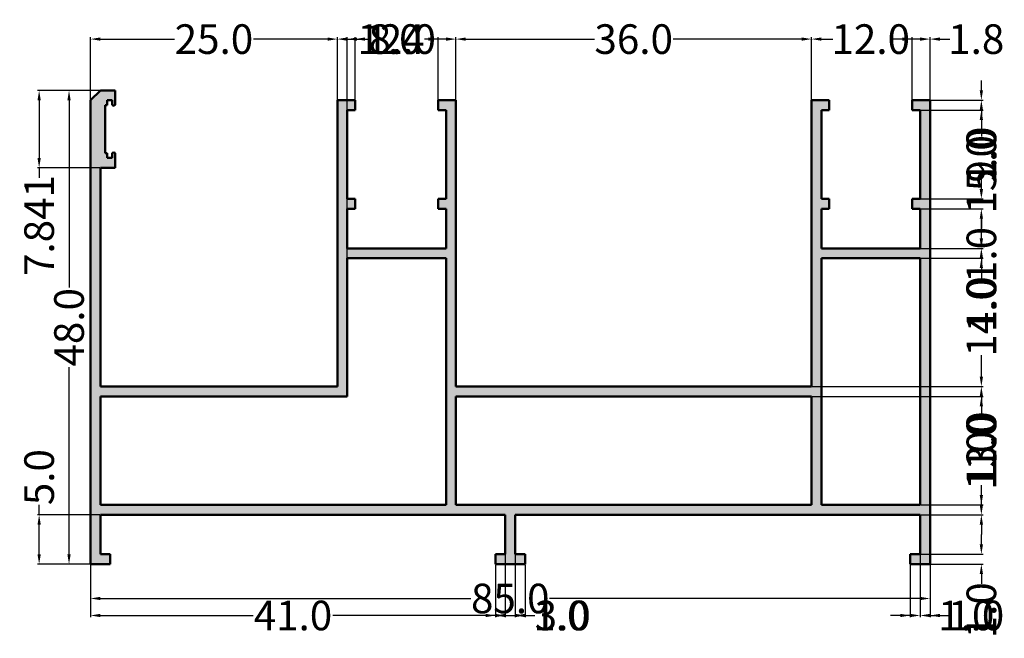
# Model space of a CAD drawing. Units: millimetres. Extents: x 9 to 262, y -226 to 104.
# Tile 2 of 4: x 9 to 109, y 42 to 104. Entities that reach past the tile are written whole.
import ezdxf

# ---------------------------------------------------------------- set-up
doc = ezdxf.new("R2010")
doc.units = ezdxf.units.MM
doc.header["$MEASUREMENT"] = 0
for name, color, linetype, lineweight in [('M-DIMS', 2, 'Continuous', 25), ('M-HATC', 9, 'Continuous', 18), ('M-OUTL', 7, 'Continuous', 50)]:
    doc.layers.add(name, color=color, linetype=linetype, lineweight=lineweight)
doc.styles.get("Standard").update_dxf_attribs({"font": 'arial.ttf'})
doc.dimstyles.get("Standard").update_dxf_attribs({"dimtxt": 3, "dimasz": 1, "dimexe": 0.18, "dimexo": 0.0625, "dimgap": 0.09, "dimtad": 0, "dimdec": 1, "dimzin": 0, "dimdsep": 46, "dimtxsty": 'Standard', "dimcen": 0.09, "dimadec": 0, "dimazin": 0, "dimtfac": 1, "dimtdec": 1, "dimtofl": 0, "dimtmove": 0, "dimatfit": 3, "dimfxl": 1, "dimtolj": 1, "dimtzin": 0, "dimarcsym": 0})

# ---------------------------------------------------------------- blocks, each defined once
blk = doc.blocks.new('*D1')
at = {"layer": 'Defpoints', "color": 0, "transparency": 16777216}
for p in [(17.228, 97.071), (14.054, 49.071), (17.228, 49.071)]:
    blk.add_point(p, dxfattribs=at)
at = {"layer": 'M-DIMS', "color": 0, "lineweight": -2, "transparency": 16777216}
for p, q in [((17.166, 97.071), (13.874, 97.071)), ((14.054, 96.071), (14.054, 77.112)), ((14.054, 50.071), (14.054, 69.029)), ((17.166, 49.071), (13.874, 49.071))]:
    blk.add_line(p, q, dxfattribs=at)
at = {"layer": 'M-DIMS', "color": 0, "transparency": 16777216}
for points in [[(13.888, 96.071), (14.221, 96.071), (14.054, 97.071)], [(13.888, 50.071), (14.221, 50.071), (14.054, 49.071)]]:
    blk.add_solid(points, dxfattribs=at)
at = {"layer": 'M-DIMS', "color": 0, "transparency": 16777216, "insert": (14.054, 73.071), "char_height": 3, "attachment_point": 5, "rotation": 90}
blk.add_mtext('\\A1;48.0', dxfattribs=at)
blk = doc.blocks.new('*D2')
at = {"layer": 'Defpoints', "color": 0, "transparency": 16777216}
for p in [(16.228, 49.071), (101.228, 49.071), (101.228, 45.592)]:
    blk.add_point(p, dxfattribs=at)
at = {"layer": 'M-DIMS', "color": 0, "lineweight": -2, "transparency": 16777216}
for p, q in [((16.228, 49.008), (16.228, 45.412)), ((101.228, 49.008), (101.228, 45.412)), ((17.228, 45.592), (54.745, 45.592)), ((100.228, 45.592), (62.711, 45.592))]:
    blk.add_line(p, q, dxfattribs=at)
at = {"layer": 'M-DIMS', "color": 0, "transparency": 16777216}
for points in [[(17.228, 45.759), (17.228, 45.426), (16.228, 45.592)], [(100.228, 45.759), (100.228, 45.426), (101.228, 45.592)]]:
    blk.add_solid(points, dxfattribs=at)
at = {"layer": 'M-DIMS', "color": 0, "transparency": 16777216, "insert": (58.728, 45.592), "char_height": 3, "attachment_point": 5}
blk.add_mtext('\\A1;85.0', dxfattribs=at)
blk = doc.blocks.new('PROFILE-FRAME')
for p, q in [((0, 47), (1, 48)), ((1, 48), (2.5, 48)), ((2.5, 48), (2.5, 46.6)), ((0, 47), (0, 0)), ((1.7, 47), (2.2, 47)), ((1.7, 47), (2.2, 47)), ((2.2, 47), (1.7, 47)), ((1.7, 47), (1.7, 46.5)), ((2.2, 46.6), (2.2, 47)), ((25, 47), (25, 18)), ((25, 47), (26.8, 47)), ((26.8, 47), (26.8, 46)), ((36, 47), (35.2, 47)), ((35.2, 47), (35.2, 46)), ((35.2, 47), (37, 47)), ((37, 47), (37, 18)), ((73, 47), (73, 18)), ((73, 47), (74.8, 47)), ((74, 47), (74.8, 47)), ((74.8, 47), (74.8, 46)), ((84, 47), (83.2, 47)), ((83.2, 47), (83.2, 46)), ((83.2, 47), (85, 47)), ((85, 47), (85, 0)), ((1.5, 46.5), (1.5, 41.659)), ((1.7, 46.5), (1.5, 46.5)), ((26, 46), (26, 37)), ((26, 46), (26.8, 46)), ((35.2, 46), (36, 46)), ((35.2, 46), (36, 46)), ((36, 46), (36, 37)), ((74, 46), (74, 37)), ((74, 46), (74.8, 46)), ((83.2, 46), (84, 46)), ((84, 46), (84, 37)), ((1.7, 41.659), (1.5, 41.659)), ((1.7, 41.159), (1.7, 41.659)), ((1.7, 41.159), (2.2, 41.159)), ((1.7, 41.159), (2.2, 41.159)), ((2.2, 41.159), (1.7, 41.159)), ((2.2, 41.559), (2.2, 41.159)), ((2.5, 40.159), (2.5, 41.559)), ((1, 40.159), (2.5, 40.159)), ((1, 40.159), (1, 18)), ((26, 37), (26.8, 37)), ((26.8, 37), (26.8, 36)), ((35.2, 37), (36, 37)), ((35.2, 37), (36, 37)), ((35.2, 37), (35.2, 36)), ((74, 37), (74.8, 37)), ((74.8, 37), (74.8, 36)), ((83.2, 37), (84, 37)), ((83.2, 37), (83.2, 36)), ((26, 36), (26.8, 36)), ((26, 36), (26, 33)), ((35.2, 36), (36, 36)), ((36, 36), (36, 33)), ((74, 36), (74.8, 36)), ((74, 36), (74, 33)), ((83.2, 36), (84, 36)), ((84, 36), (84, 33)), ((26, 33), (26, 32)), ((36, 33), (36, 32)), ((74, 33), (74, 32)), ((84, 33), (84, 32)), ((26, 32), (36, 32)), ((74, 32), (84, 32)), ((26, 31), (36, 31)), ((26, 31), (26, 27)), ((36, 31), (36, 27)), ((74, 31), (84, 31)), ((74, 31), (74, 27)), ((84, 31), (84, 27)), ((26, 27), (26, 17)), ((36, 27), (36, 6)), ((74, 27), (74, 17)), ((84, 27), (84, 17)), ((1, 18), (25, 18)), ((37, 18), (73, 18)), ((1, 17), (26, 17)), ((1, 17), (1, 6)), ((37, 17), (73, 17)), ((37, 17), (37, 6)), ((73, 17), (73, 6)), ((74, 17), (74, 6)), ((84, 17), (84, 6)), ((1, 6), (36, 6)), ((37, 6), (73, 6)), ((74, 6), (84, 6)), ((1, 5), (42, 5)), ((1, 5), (1, 1)), ((42, 5), (42, 1)), ((43, 5), (43, 1)), ((43, 5), (84, 5)), ((84, 5), (84, 1)), ((1, 1), (2, 1)), ((1, 1), (2, 1)), ((2, 1), (2, 0)), ((41, 1), (42, 1)), ((41, 1), (41, 0)), ((43, 1), (44, 1)), ((43, 1), (44, 1)), ((44, 1), (44, 0)), ((84, 1), (83, 1)), ((83, 1), (83, 0)), ((83, 1), (84, 1)), ((0, 0), (2, 0)), ((41, 0), (44, 0)), ((83, 0), (85, 0))]:
    blk.add_line(p, q)
for centre, start, end in [((2.35, 46.6), 180, 0), ((2.35, 41.559), 0, 180)]:
    blk.add_arc(centre, 0.15, start, end)
blk = doc.blocks.new('*D7')
at = {"layer": 'Defpoints', "color": 0, "transparency": 16777216}
for p in [(41.228, 102.271), (16.228, 96.071), (41.228, 96.071)]:
    blk.add_point(p, dxfattribs=at)
at = {"layer": 'M-DIMS', "color": 0, "lineweight": -2, "transparency": 16777216}
for p, q in [((16.228, 96.133), (16.228, 102.451)), ((17.228, 102.271), (24.721, 102.271)), ((40.228, 102.271), (32.735, 102.271)), ((41.228, 96.133), (41.228, 102.451))]:
    blk.add_line(p, q, dxfattribs=at)
at = {"layer": 'M-DIMS', "color": 0, "transparency": 16777216}
for points in [[(17.228, 102.438), (17.228, 102.104), (16.228, 102.271)], [(40.228, 102.438), (40.228, 102.104), (41.228, 102.271)]]:
    blk.add_solid(points, dxfattribs=at)
at = {"layer": 'M-DIMS', "color": 0, "transparency": 16777216, "insert": (28.728, 102.271), "char_height": 3, "attachment_point": 5}
blk.add_mtext('\\A1;25.0', dxfattribs=at)
blk = doc.blocks.new('*D8')
at = {"layer": 'Defpoints', "color": 0, "transparency": 16777216}
for p in [(53.228, 102.271), (41.228, 96.071), (53.228, 96.071)]:
    blk.add_point(p, dxfattribs=at)
at = {"layer": 'M-DIMS', "color": 0, "lineweight": -2, "transparency": 16777216}
for p, q in [((41.228, 96.133), (41.228, 102.451)), ((42.228, 102.271), (43.388, 102.271)), ((52.228, 102.271), (51.068, 102.271)), ((53.228, 96.133), (53.228, 102.451))]:
    blk.add_line(p, q, dxfattribs=at)
at = {"layer": 'M-DIMS', "color": 0, "transparency": 16777216}
for points in [[(42.228, 102.438), (42.228, 102.104), (41.228, 102.271)], [(52.228, 102.438), (52.228, 102.104), (53.228, 102.271)]]:
    blk.add_solid(points, dxfattribs=at)
at = {"layer": 'M-DIMS', "color": 0, "transparency": 16777216, "insert": (47.228, 102.271), "char_height": 3, "attachment_point": 5}
blk.add_mtext('\\A1;12.0', dxfattribs=at)
blk = doc.blocks.new('*D9')
at = {"layer": 'Defpoints', "color": 0, "transparency": 16777216}
for p in [(89.228, 102.271), (53.228, 96.071), (89.228, 96.071)]:
    blk.add_point(p, dxfattribs=at)
at = {"layer": 'M-DIMS', "color": 0, "lineweight": -2, "transparency": 16777216}
for p, q in [((53.228, 96.133), (53.228, 102.451)), ((54.228, 102.271), (67.248, 102.271)), ((88.228, 102.271), (75.208, 102.271)), ((89.228, 96.133), (89.228, 102.451))]:
    blk.add_line(p, q, dxfattribs=at)
at = {"layer": 'M-DIMS', "color": 0, "transparency": 16777216}
for points in [[(54.228, 102.438), (54.228, 102.104), (53.228, 102.271)], [(88.228, 102.438), (88.228, 102.104), (89.228, 102.271)]]:
    blk.add_solid(points, dxfattribs=at)
at = {"layer": 'M-DIMS', "color": 0, "transparency": 16777216, "insert": (71.228, 102.271), "char_height": 3, "attachment_point": 5}
blk.add_mtext('\\A1;36.0', dxfattribs=at)
blk = doc.blocks.new('*D10')
at = {"layer": 'Defpoints', "color": 0, "transparency": 16777216}
for p in [(101.228, 102.271), (89.228, 96.071), (101.228, 96.071)]:
    blk.add_point(p, dxfattribs=at)
at = {"layer": 'M-DIMS', "color": 0, "lineweight": -2, "transparency": 16777216}
for p, q in [((89.228, 96.133), (89.228, 102.451)), ((90.228, 102.271), (91.388, 102.271)), ((100.228, 102.271), (99.068, 102.271)), ((101.228, 96.133), (101.228, 102.451))]:
    blk.add_line(p, q, dxfattribs=at)
at = {"layer": 'M-DIMS', "color": 0, "transparency": 16777216}
for points in [[(90.228, 102.438), (90.228, 102.104), (89.228, 102.271)], [(100.228, 102.438), (100.228, 102.104), (101.228, 102.271)]]:
    blk.add_solid(points, dxfattribs=at)
at = {"layer": 'M-DIMS', "color": 0, "transparency": 16777216, "insert": (95.228, 102.271), "char_height": 3, "attachment_point": 5}
blk.add_mtext('\\A1;12.0', dxfattribs=at)
blk = doc.blocks.new('*D11')
at = {"layer": 'Defpoints', "color": 0, "transparency": 16777216}
for p in [(11.028, 54.071), (17.228, 54.071), (16.228, 49.071)]:
    blk.add_point(p, dxfattribs=at)
at = {"layer": 'M-DIMS', "color": 0, "lineweight": -2, "transparency": 16777216}
for p, q in [((11.028, 54.071), (11.028, 55.071)), ((17.166, 54.071), (10.848, 54.071)), ((11.028, 50.071), (11.028, 53.071)), ((16.166, 49.071), (10.848, 49.071))]:
    blk.add_line(p, q, dxfattribs=at)
at = {"layer": 'M-DIMS', "color": 0, "transparency": 16777216}
for points in [[(10.861, 53.071), (11.195, 53.071), (11.028, 54.071)], [(10.861, 50.071), (11.195, 50.071), (11.028, 49.071)]]:
    blk.add_solid(points, dxfattribs=at)
at = {"layer": 'M-DIMS', "color": 0, "transparency": 16777216, "insert": (11.028, 57.887), "char_height": 3, "attachment_point": 5, "rotation": 90}
blk.add_mtext('\\A1;5.0', dxfattribs=at)
blk = doc.blocks.new('*D12')
at = {"layer": 'Defpoints', "color": 0, "transparency": 16777216}
for p in [(89.228, 67.071), (106.428, 67.071), (100.228, 54.071)]:
    blk.add_point(p, dxfattribs=at)
at = {"layer": 'M-DIMS', "color": 0, "lineweight": -2, "transparency": 16777216}
for p, q in [((89.291, 67.071), (106.608, 67.071)), ((106.428, 66.071), (106.428, 64.411)), ((106.428, 55.071), (106.428, 56.731)), ((100.291, 54.071), (106.608, 54.071))]:
    blk.add_line(p, q, dxfattribs=at)
at = {"layer": 'M-DIMS', "color": 0, "transparency": 16777216}
for points in [[(106.261, 66.071), (106.595, 66.071), (106.428, 67.071)], [(106.261, 55.071), (106.595, 55.071), (106.428, 54.071)]]:
    blk.add_solid(points, dxfattribs=at)
at = {"layer": 'M-DIMS', "color": 0, "transparency": 16777216, "insert": (106.428, 60.571), "char_height": 3, "attachment_point": 5, "rotation": 90}
blk.add_mtext('\\A1;13.0', dxfattribs=at)
blk = doc.blocks.new('*D13')
at = {"layer": 'Defpoints', "color": 0, "transparency": 16777216}
for p in [(90.228, 81.071), (106.428, 81.071), (89.228, 67.071)]:
    blk.add_point(p, dxfattribs=at)
at = {"layer": 'M-DIMS', "color": 0, "lineweight": -2, "transparency": 16777216}
for p, q in [((90.291, 81.071), (106.608, 81.071)), ((106.428, 80.071), (106.428, 77.911)), ((106.428, 68.071), (106.428, 70.231)), ((89.291, 67.071), (106.608, 67.071))]:
    blk.add_line(p, q, dxfattribs=at)
at = {"layer": 'M-DIMS', "color": 0, "transparency": 16777216}
for points in [[(106.261, 80.071), (106.595, 80.071), (106.428, 81.071)], [(106.261, 68.071), (106.595, 68.071), (106.428, 67.071)]]:
    blk.add_solid(points, dxfattribs=at)
at = {"layer": 'M-DIMS', "color": 0, "transparency": 16777216, "insert": (106.428, 74.071), "char_height": 3, "attachment_point": 5, "rotation": 90}
blk.add_mtext('\\A1;14.0', dxfattribs=at)
blk = doc.blocks.new('*D14')
at = {"layer": 'Defpoints', "color": 0, "transparency": 16777216}
for p in [(101.228, 96.071), (106.428, 96.071), (90.228, 81.071)]:
    blk.add_point(p, dxfattribs=at)
at = {"layer": 'M-DIMS', "color": 0, "lineweight": -2, "transparency": 16777216}
for p, q in [((101.291, 96.071), (106.608, 96.071)), ((106.428, 95.071), (106.428, 92.411)), ((106.428, 82.071), (106.428, 84.731)), ((90.291, 81.071), (106.608, 81.071))]:
    blk.add_line(p, q, dxfattribs=at)
at = {"layer": 'M-DIMS', "color": 0, "transparency": 16777216}
for points in [[(106.261, 95.071), (106.595, 95.071), (106.428, 96.071)], [(106.261, 82.071), (106.595, 82.071), (106.428, 81.071)]]:
    blk.add_solid(points, dxfattribs=at)
at = {"layer": 'M-DIMS', "color": 0, "transparency": 16777216, "insert": (106.428, 88.571), "char_height": 3, "attachment_point": 5, "rotation": 90}
blk.add_mtext('\\A1;15.0', dxfattribs=at)
blk = doc.blocks.new('*D15')
at = {"layer": 'Defpoints', "color": 0, "transparency": 16777216}
for p in [(16.228, 49.071), (57.228, 49.071), (57.228, 43.871)]:
    blk.add_point(p, dxfattribs=at)
at = {"layer": 'M-DIMS', "color": 0, "lineweight": -2, "transparency": 16777216}
for p, q in [((16.228, 49.008), (16.228, 43.691)), ((57.228, 49.008), (57.228, 43.691)), ((17.228, 43.871), (32.687, 43.871)), ((56.228, 43.871), (40.77, 43.871))]:
    blk.add_line(p, q, dxfattribs=at)
at = {"layer": 'M-DIMS', "color": 0, "transparency": 16777216}
for points in [[(17.228, 44.038), (17.228, 43.704), (16.228, 43.871)], [(56.228, 44.038), (56.228, 43.704), (57.228, 43.871)]]:
    blk.add_solid(points, dxfattribs=at)
at = {"layer": 'M-DIMS', "color": 0, "transparency": 16777216, "insert": (36.728, 43.871), "char_height": 3, "attachment_point": 5}
blk.add_mtext('\\A1;41.0', dxfattribs=at)
blk = doc.blocks.new('*D16')
at = {"layer": 'Defpoints', "color": 0, "transparency": 16777216}
for p in [(57.228, 49.071), (60.228, 49.071), (60.228, 43.871)]:
    blk.add_point(p, dxfattribs=at)
at = {"layer": 'M-DIMS', "color": 0, "lineweight": -2, "transparency": 16777216}
for p, q in [((57.228, 49.008), (57.228, 43.691)), ((60.228, 49.008), (60.228, 43.691)), ((58.228, 43.871), (59.228, 43.871)), ((60.228, 43.871), (61.228, 43.871))]:
    blk.add_line(p, q, dxfattribs=at)
at = {"layer": 'M-DIMS', "color": 0, "transparency": 16777216}
for points in [[(58.228, 44.038), (58.228, 43.704), (57.228, 43.871)], [(59.228, 44.038), (59.228, 43.704), (60.228, 43.871)]]:
    blk.add_solid(points, dxfattribs=at)
at = {"layer": 'M-DIMS', "color": 0, "transparency": 16777216, "insert": (64.043, 43.871), "char_height": 3, "attachment_point": 5}
blk.add_mtext('\\A1;3.0', dxfattribs=at)
blk = doc.blocks.new('*D17')
at = {"layer": 'Defpoints', "color": 0, "transparency": 16777216}
for p in [(100.228, 54.071), (101.228, 49.071), (101.228, 43.871)]:
    blk.add_point(p, dxfattribs=at)
at = {"layer": 'M-DIMS', "color": 0, "lineweight": -2, "transparency": 16777216}
for p, q in [((100.228, 54.008), (100.228, 43.691)), ((101.228, 49.008), (101.228, 43.691)), ((99.228, 43.871), (98.228, 43.871)), ((102.228, 43.871), (103.228, 43.871))]:
    blk.add_line(p, q, dxfattribs=at)
at = {"layer": 'M-DIMS', "color": 0, "transparency": 16777216}
for points in [[(99.228, 44.038), (99.228, 43.704), (100.228, 43.871)], [(102.228, 44.038), (102.228, 43.704), (101.228, 43.871)]]:
    blk.add_solid(points, dxfattribs=at)
at = {"layer": 'M-DIMS', "color": 0, "transparency": 16777216, "insert": (105.903, 43.871), "char_height": 3, "attachment_point": 5}
blk.add_mtext('\\A1;1.0', dxfattribs=at)
blk = doc.blocks.new('*D18')
at = {"layer": 'Defpoints', "color": 0, "transparency": 16777216}
for p in [(51.428, 102.271), (43.028, 95.071), (51.428, 95.071)]:
    blk.add_point(p, dxfattribs=at)
at = {"layer": 'M-DIMS', "color": 0, "lineweight": -2, "transparency": 16777216}
for p, q in [((43.028, 95.133), (43.028, 102.451)), ((44.028, 102.271), (44.411, 102.271)), ((50.428, 102.271), (50.045, 102.271)), ((51.428, 95.133), (51.428, 102.451))]:
    blk.add_line(p, q, dxfattribs=at)
at = {"layer": 'M-DIMS', "color": 0, "transparency": 16777216}
for points in [[(44.028, 102.438), (44.028, 102.104), (43.028, 102.271)], [(50.428, 102.438), (50.428, 102.104), (51.428, 102.271)]]:
    blk.add_solid(points, dxfattribs=at)
at = {"layer": 'M-DIMS', "color": 0, "transparency": 16777216, "insert": (47.228, 102.271), "char_height": 3, "attachment_point": 5}
blk.add_mtext('\\A1;8.4', dxfattribs=at)
blk = doc.blocks.new('*D19')
at = {"layer": 'Defpoints', "color": 0, "transparency": 16777216}
for p in [(18.728, 97.071), (11.028, 89.23), (17.228, 89.23)]:
    blk.add_point(p, dxfattribs=at)
at = {"layer": 'M-DIMS', "color": 0, "lineweight": -2, "transparency": 16777216}
for p, q in [((18.666, 97.071), (10.848, 97.071)), ((11.028, 96.071), (11.028, 90.23)), ((17.166, 89.23), (10.848, 89.23)), ((11.028, 89.23), (11.028, 88.23))]:
    blk.add_line(p, q, dxfattribs=at)
at = {"layer": 'M-DIMS', "color": 0, "transparency": 16777216}
for points in [[(10.861, 96.071), (11.195, 96.071), (11.028, 97.071)], [(10.861, 90.23), (11.195, 90.23), (11.028, 89.23)]]:
    blk.add_solid(points, dxfattribs=at)
at = {"layer": 'M-DIMS', "color": 0, "transparency": 16777216, "insert": (11.028, 83.38), "char_height": 3, "attachment_point": 5, "rotation": 90}
blk.add_mtext('\\A1;7.841', dxfattribs=at)
blk = doc.blocks.new('*D35')
at = {"layer": 'Defpoints', "color": 0, "transparency": 16777216}
for p in [(100.228, 55.071), (106.428, 55.071), (100.228, 54.071)]:
    blk.add_point(p, dxfattribs=at)
at = {"layer": 'M-DIMS', "color": 0, "lineweight": -2, "transparency": 16777216}
for p, q in [((106.428, 56.071), (106.428, 57.071)), ((100.291, 55.071), (106.608, 55.071)), ((100.291, 54.071), (106.608, 54.071)), ((106.428, 53.071), (106.428, 52.071))]:
    blk.add_line(p, q, dxfattribs=at)
at = {"layer": 'M-DIMS', "color": 0, "transparency": 16777216}
for points in [[(106.261, 56.071), (106.595, 56.071), (106.428, 55.071)], [(106.261, 53.071), (106.595, 53.071), (106.428, 54.071)]]:
    blk.add_solid(points, dxfattribs=at)
at = {"layer": 'M-DIMS', "color": 0, "transparency": 16777216, "insert": (106.428, 59.746), "char_height": 3, "attachment_point": 5, "rotation": 90}
blk.add_mtext('\\A1;1.0', dxfattribs=at)
blk = doc.blocks.new('*D36')
at = {"layer": 'Defpoints', "color": 0, "transparency": 16777216}
for p in [(89.228, 67.071), (89.228, 66.071), (106.428, 66.071)]:
    blk.add_point(p, dxfattribs=at)
at = {"layer": 'M-DIMS', "color": 0, "lineweight": -2, "transparency": 16777216}
for p, q in [((106.428, 68.071), (106.428, 69.071)), ((89.291, 67.071), (106.608, 67.071)), ((89.291, 66.071), (106.608, 66.071)), ((106.428, 65.071), (106.428, 64.071))]:
    blk.add_line(p, q, dxfattribs=at)
at = {"layer": 'M-DIMS', "color": 0, "transparency": 16777216}
for points in [[(106.261, 68.071), (106.595, 68.071), (106.428, 67.071)], [(106.261, 65.071), (106.595, 65.071), (106.428, 66.071)]]:
    blk.add_solid(points, dxfattribs=at)
at = {"layer": 'M-DIMS', "color": 0, "transparency": 16777216, "insert": (106.428, 61.396), "char_height": 3, "attachment_point": 5, "rotation": 90}
blk.add_mtext('\\A1;1.0', dxfattribs=at)
blk = doc.blocks.new('*D37')
at = {"layer": 'Defpoints', "color": 0, "transparency": 16777216}
for p in [(90.228, 81.071), (90.228, 80.071), (106.428, 80.071)]:
    blk.add_point(p, dxfattribs=at)
at = {"layer": 'M-DIMS', "color": 0, "lineweight": -2, "transparency": 16777216}
for p, q in [((106.428, 82.071), (106.428, 83.071)), ((90.291, 81.071), (106.608, 81.071)), ((90.291, 80.071), (106.608, 80.071)), ((106.428, 79.071), (106.428, 78.071))]:
    blk.add_line(p, q, dxfattribs=at)
at = {"layer": 'M-DIMS', "color": 0, "transparency": 16777216}
for points in [[(106.261, 82.071), (106.595, 82.071), (106.428, 81.071)], [(106.261, 79.071), (106.595, 79.071), (106.428, 80.071)]]:
    blk.add_solid(points, dxfattribs=at)
at = {"layer": 'M-DIMS', "color": 0, "transparency": 16777216, "insert": (106.428, 75.396), "char_height": 3, "attachment_point": 5, "rotation": 90}
blk.add_mtext('\\A1;1.0', dxfattribs=at)
blk = doc.blocks.new('*D38')
at = {"layer": 'Defpoints', "color": 0, "transparency": 16777216}
for p in [(42.228, 102.271), (41.228, 67.071), (42.228, 66.071)]:
    blk.add_point(p, dxfattribs=at)
at = {"layer": 'M-DIMS', "color": 0, "lineweight": -2, "transparency": 16777216}
for p, q in [((40.228, 102.271), (39.228, 102.271)), ((41.228, 67.133), (41.228, 102.451)), ((42.228, 66.133), (42.228, 102.451)), ((43.228, 102.271), (44.228, 102.271))]:
    blk.add_line(p, q, dxfattribs=at)
at = {"layer": 'M-DIMS', "color": 0, "transparency": 16777216}
for points in [[(40.228, 102.438), (40.228, 102.104), (41.228, 102.271)], [(43.228, 102.438), (43.228, 102.104), (42.228, 102.271)]]:
    blk.add_solid(points, dxfattribs=at)
at = {"layer": 'M-DIMS', "color": 0, "transparency": 16777216, "insert": (46.903, 102.271), "char_height": 3, "attachment_point": 5}
blk.add_mtext('\\A1;1.0', dxfattribs=at)
blk = doc.blocks.new('*D39')
at = {"layer": 'Defpoints', "color": 0, "transparency": 16777216}
for p in [(58.228, 54.071), (59.228, 54.071), (59.228, 43.871)]:
    blk.add_point(p, dxfattribs=at)
at = {"layer": 'M-DIMS', "color": 0, "lineweight": -2, "transparency": 16777216}
for p, q in [((58.228, 54.008), (58.228, 43.691)), ((59.228, 54.008), (59.228, 43.691)), ((57.228, 43.871), (56.228, 43.871)), ((60.228, 43.871), (61.228, 43.871))]:
    blk.add_line(p, q, dxfattribs=at)
at = {"layer": 'M-DIMS', "color": 0, "transparency": 16777216}
for points in [[(57.228, 44.038), (57.228, 43.704), (58.228, 43.871)], [(60.228, 44.038), (60.228, 43.704), (59.228, 43.871)]]:
    blk.add_solid(points, dxfattribs=at)
at = {"layer": 'M-DIMS', "color": 0, "transparency": 16777216, "insert": (63.903, 43.871), "char_height": 3, "attachment_point": 5}
blk.add_mtext('\\A1;1.0', dxfattribs=at)
blk = doc.blocks.new('*D40')
at = {"layer": 'Defpoints', "color": 0, "transparency": 16777216}
for p in [(99.228, 50.071), (99.228, 49.071), (106.428, 49.071)]:
    blk.add_point(p, dxfattribs=at)
at = {"layer": 'M-DIMS', "color": 0, "lineweight": -2, "transparency": 16777216}
for p, q in [((106.428, 51.071), (106.428, 52.071)), ((99.291, 50.071), (106.608, 50.071)), ((99.291, 49.071), (106.608, 49.071)), ((106.428, 48.071), (106.428, 47.071))]:
    blk.add_line(p, q, dxfattribs=at)
at = {"layer": 'M-DIMS', "color": 0, "transparency": 16777216}
for points in [[(106.261, 51.071), (106.595, 51.071), (106.428, 50.071)], [(106.261, 48.071), (106.595, 48.071), (106.428, 49.071)]]:
    blk.add_solid(points, dxfattribs=at)
at = {"layer": 'M-DIMS', "color": 0, "transparency": 16777216, "insert": (106.428, 44.396), "char_height": 3, "attachment_point": 5, "rotation": 90}
blk.add_mtext('\\A1;1.0', dxfattribs=at)
blk = doc.blocks.new('*D41')
at = {"layer": 'Defpoints', "color": 0, "transparency": 16777216}
for p in [(100.228, 50.071), (99.228, 49.071), (100.228, 43.871)]:
    blk.add_point(p, dxfattribs=at)
at = {"layer": 'M-DIMS', "color": 0, "lineweight": -2, "transparency": 16777216}
for p, q in [((100.228, 50.008), (100.228, 43.691)), ((99.228, 49.008), (99.228, 43.691)), ((98.228, 43.871), (97.228, 43.871)), ((101.228, 43.871), (102.228, 43.871))]:
    blk.add_line(p, q, dxfattribs=at)
at = {"layer": 'M-DIMS', "color": 0, "transparency": 16777216}
for points in [[(98.228, 44.038), (98.228, 43.704), (99.228, 43.871)], [(101.228, 44.038), (101.228, 43.704), (100.228, 43.871)]]:
    blk.add_solid(points, dxfattribs=at)
at = {"layer": 'M-DIMS', "color": 0, "transparency": 16777216, "insert": (104.903, 43.871), "char_height": 3, "attachment_point": 5}
blk.add_mtext('\\A1;1.0', dxfattribs=at)
blk = doc.blocks.new('*D42')
at = {"layer": 'Defpoints', "color": 0, "transparency": 16777216}
for p in [(101.228, 102.271), (99.428, 96.071), (101.228, 96.071)]:
    blk.add_point(p, dxfattribs=at)
at = {"layer": 'M-DIMS', "color": 0, "lineweight": -2, "transparency": 16777216}
for p, q in [((98.428, 102.271), (97.428, 102.271)), ((99.428, 96.133), (99.428, 102.451)), ((101.228, 96.133), (101.228, 102.451)), ((102.228, 102.271), (103.228, 102.271))]:
    blk.add_line(p, q, dxfattribs=at)
at = {"layer": 'M-DIMS', "color": 0, "transparency": 16777216}
for points in [[(98.428, 102.438), (98.428, 102.104), (99.428, 102.271)], [(102.228, 102.438), (102.228, 102.104), (101.228, 102.271)]]:
    blk.add_solid(points, dxfattribs=at)
at = {"layer": 'M-DIMS', "color": 0, "transparency": 16777216, "insert": (105.911, 102.271), "char_height": 3, "attachment_point": 5}
blk.add_mtext('\\A1;1.8', dxfattribs=at)
blk = doc.blocks.new('*D43')
at = {"layer": 'Defpoints', "color": 0, "transparency": 16777216}
for p in [(99.428, 96.071), (99.428, 95.071), (106.428, 95.071)]:
    blk.add_point(p, dxfattribs=at)
at = {"layer": 'M-DIMS', "color": 0, "lineweight": -2, "transparency": 16777216}
for p, q in [((106.428, 97.071), (106.428, 98.071)), ((99.491, 96.071), (106.608, 96.071)), ((99.491, 95.071), (106.608, 95.071)), ((106.428, 94.071), (106.428, 93.071))]:
    blk.add_line(p, q, dxfattribs=at)
at = {"layer": 'M-DIMS', "color": 0, "transparency": 16777216}
for points in [[(106.261, 97.071), (106.595, 97.071), (106.428, 96.071)], [(106.261, 94.071), (106.595, 94.071), (106.428, 95.071)]]:
    blk.add_solid(points, dxfattribs=at)
at = {"layer": 'M-DIMS', "color": 0, "transparency": 16777216, "insert": (106.428, 90.396), "char_height": 3, "attachment_point": 5, "rotation": 90}
blk.add_mtext('\\A1;1.0', dxfattribs=at)
blk = doc.blocks.new('*D44')
at = {"layer": 'Defpoints', "color": 0, "transparency": 16777216}
for p in [(99.428, 95.071), (99.428, 86.071), (106.428, 86.071)]:
    blk.add_point(p, dxfattribs=at)
at = {"layer": 'M-DIMS', "color": 0, "lineweight": -2, "transparency": 16777216}
for p, q in [((99.491, 95.071), (106.608, 95.071)), ((106.428, 94.071), (106.428, 93.387)), ((106.428, 87.071), (106.428, 87.755)), ((99.491, 86.071), (106.608, 86.071))]:
    blk.add_line(p, q, dxfattribs=at)
at = {"layer": 'M-DIMS', "color": 0, "transparency": 16777216}
for points in [[(106.261, 94.071), (106.595, 94.071), (106.428, 95.071)], [(106.261, 87.071), (106.595, 87.071), (106.428, 86.071)]]:
    blk.add_solid(points, dxfattribs=at)
at = {"layer": 'M-DIMS', "color": 0, "transparency": 16777216, "insert": (106.428, 90.571), "char_height": 3, "attachment_point": 5, "rotation": 90}
blk.add_mtext('\\A1;9.0', dxfattribs=at)
blk = doc.blocks.new('*D45')
at = {"layer": 'Defpoints', "color": 0, "transparency": 16777216}
for p in [(99.428, 86.071), (99.428, 85.071), (106.428, 85.071)]:
    blk.add_point(p, dxfattribs=at)
at = {"layer": 'M-DIMS', "color": 0, "lineweight": -2, "transparency": 16777216}
for p, q in [((106.428, 87.071), (106.428, 88.071)), ((99.491, 86.071), (106.608, 86.071)), ((99.491, 85.071), (106.608, 85.071)), ((106.428, 84.071), (106.428, 83.071))]:
    blk.add_line(p, q, dxfattribs=at)
at = {"layer": 'M-DIMS', "color": 0, "transparency": 16777216}
for points in [[(106.261, 87.071), (106.595, 87.071), (106.428, 86.071)], [(106.261, 84.071), (106.595, 84.071), (106.428, 85.071)]]:
    blk.add_solid(points, dxfattribs=at)
at = {"layer": 'M-DIMS', "color": 0, "transparency": 16777216, "insert": (106.428, 80.396), "char_height": 3, "attachment_point": 5, "rotation": 90}
blk.add_mtext('\\A1;1.0', dxfattribs=at)

msp = doc.modelspace()

# ---------------------------------------------------------------- hatches: boundary and pattern name
at = {"layer": 'M-HATC'}
h = msp.add_hatch(color=256, dxfattribs=at)
h.dxf.hatch_style = 1
h.paths.add_polyline_path([(53.2282, 96.0709), (51.4282, 96.0709), (51.4282, 95.0709), (52.2282, 95.0709), (52.2282, 86.0709), (51.4282, 86.0709), (51.4282, 85.0709), (52.2282, 85.0709), (52.2282, 82.0709), (52.2282, 81.0709), (42.2282, 81.0709), (42.2282, 82.0709), (42.2282, 85.0709), (43.0282, 85.0709), (43.0282, 86.0709), (42.2282, 86.0709), (42.2282, 95.0709), (43.0282, 95.0709), (43.0282, 96.0709), (41.2282, 96.0709), (41.2282, 67.0709), (17.2282, 67.0709), (17.2282, 89.23), (18.7282, 89.23), (18.7282, 90.63, 1), (18.4282, 90.63), (18.4282, 90.23), (17.9282, 90.23), (17.9282, 90.73), (17.7282, 90.73), (17.7282, 95.5709), (17.9282, 95.5709), (17.9282, 96.0709), (18.4282, 96.0709), (18.4282, 95.6709, 1), (18.7282, 95.6709), (18.7282, 97.0709), (17.2282, 97.0709), (16.2282, 96.0709), (16.2282, 49.0709), (18.2282, 49.0709), (18.2282, 50.0709), (17.2282, 50.0709), (17.2282, 54.0709), (58.2282, 54.0709), (58.2282, 50.0709), (57.2282, 50.0709), (57.2282, 49.0709), (60.2282, 49.0709), (60.2282, 50.0709), (59.2282, 50.0709), (59.2282, 54.0709), (100.2282, 54.0709), (100.2282, 50.0709), (99.2282, 50.0709), (99.2282, 49.0709), (101.2282, 49.0709), (101.2282, 96.0709), (99.4282, 96.0709), (99.4282, 95.0709), (100.2282, 95.0709), (100.2282, 86.0709), (99.4282, 86.0709), (99.4282, 85.0709), (100.2282, 85.0709), (100.2282, 82.0709), (100.2282, 81.0709), (90.2282, 81.0709), (90.2282, 82.0709), (90.2282, 85.0709), (91.0282, 85.0709), (91.0282, 86.0709), (90.2282, 86.0709), (90.2282, 95.0709), (91.0282, 95.0709), (91.0282, 96.0709), (90.2282, 96.0709), (89.2282, 96.0709), (89.2282, 67.0709), (53.2282, 67.0709)])
h.paths.add_polyline_path([(52.2282, 80.0709), (52.2282, 76.0709), (52.2282, 55.0709), (17.2282, 55.0709), (17.2282, 66.0709), (42.2282, 66.0709), (42.2282, 76.0709), (42.2282, 80.0709)], flags=16)
h.paths.add_polyline_path([(53.2282, 66.0709), (89.2282, 66.0709), (89.2282, 55.0709), (53.2282, 55.0709)], flags=16)
h.paths.add_polyline_path([(90.2282, 80.0709), (100.2282, 80.0709), (100.2282, 76.0709), (100.2282, 66.0709), (100.2282, 55.0709), (90.2282, 55.0709), (90.2282, 66.0709), (90.2282, 76.0709)], flags=16)

# ---------------------------------------------------------------- block references
at = {"layer": 'M-OUTL'}
msp.add_blockref('PROFILE-FRAME', (16.228, 49.071), dxfattribs=at)

# ---------------------------------------------------------------- dimensions: what is measured, and where the dimension line sits
at = {"layer": 'M-DIMS'}
for base, p1, p2, override, picture, middle in [((41.2282, 102.2709), (16.2282, 96.0709), (41.2282, 96.0709), {"dimdec": 1, "dimlfac": 1, "dimrnd": 0, "dimzin": 0, "dimdsep": 46, "dimlunit": 2}, '*D7', (28.7282, 102.2709)), ((42.2282, 102.2709), (41.2282, 67.0709), (42.2282, 66.0709), {"dimdec": 1, "dimlfac": 1, "dimrnd": 0, "dimzin": 0, "dimdsep": 46, "dimlunit": 2}, '*D38', (46.9027, 102.2709)), ((53.2282, 102.2709), (41.2282, 96.0709), (53.2282, 96.0709), {"dimdec": 1, "dimlfac": 1, "dimrnd": 0, "dimzin": 0, "dimdsep": 46, "dimlunit": 2}, '*D8', (47.2282, 102.2709)), ((51.4282, 102.2709), (43.0282, 95.0709), (51.4282, 95.0709), {"dimdec": 1, "dimlfac": 1, "dimrnd": 0, "dimzin": 0, "dimdsep": 46, "dimlunit": 2}, '*D18', (47.2282, 102.2709)), ((89.2282, 102.2709), (53.2282, 96.0709), (89.2282, 96.0709), {"dimdec": 1, "dimlfac": 1, "dimrnd": 0, "dimzin": 0, "dimdsep": 46, "dimlunit": 2}, '*D9', (71.2282, 102.2709)), ((101.2282, 102.2709), (89.2282, 96.0709), (101.2282, 96.0709), {"dimdec": 1, "dimlfac": 1, "dimrnd": 0, "dimzin": 0, "dimdsep": 46, "dimlunit": 2}, '*D10', (95.2282, 102.2709)), ((101.2282, 102.2709), (99.4282, 96.0709), (101.2282, 96.0709), {"dimdec": 1, "dimlfac": 1, "dimrnd": 0, "dimzin": 0, "dimdsep": 46, "dimlunit": 2}, '*D42', (105.9109, 102.2709)), ((59.2282, 43.8709), (58.2282, 54.0709), (59.2282, 54.0709), {"dimdec": 1, "dimlfac": 1, "dimrnd": 0, "dimzin": 0, "dimdsep": 46, "dimlunit": 2}, '*D39', (63.9027, 43.8709)), ((101.2282, 43.8709), (100.2282, 54.0709), (101.2282, 49.0709), {"dimdec": 1, "dimlfac": 1, "dimrnd": 0, "dimzin": 0, "dimdsep": 46, "dimlunit": 2}, '*D17', (105.9027, 43.8709)), ((100.2282, 43.8709), (99.2282, 49.0709), (100.2282, 50.0709), {"dimdec": 1, "dimlfac": 1, "dimrnd": 0, "dimzin": 0, "dimdsep": 46, "dimlunit": 2}, '*D41', (104.9027, 43.8709)), ((101.2282, 45.5925), (16.2282, 49.0709), (101.2282, 49.0709), {"dimclrd": 0, "dimclre": 0, "dimclrt": 0}, '*D2', (58.7282, 45.5925)), ((57.2282, 43.8709), (16.2282, 49.0709), (57.2282, 49.0709), {"dimdec": 1, "dimlfac": 1, "dimrnd": 0, "dimzin": 0, "dimdsep": 46, "dimlunit": 2}, '*D15', (36.7282, 43.8709)), ((60.2282, 43.8709), (57.2282, 49.0709), (60.2282, 49.0709), {"dimdec": 1, "dimlfac": 1, "dimrnd": 0, "dimzin": 0, "dimdsep": 46, "dimlunit": 2}, '*D16', (64.0429, 43.8709))]:
    dim = msp.add_linear_dim(base=base, p1=p1, p2=p2, dimstyle='Standard', override=override, dxfattribs=at)
    dim.commit()
    dim.dimension.update_dxf_attribs({"geometry": picture, "text_midpoint": middle})
for base, p1, p2, override, picture, middle in [((106.4282, 95.0709), (99.4282, 96.0709), (99.4282, 95.0709), {"dimdec": 1, "dimlfac": 1, "dimrnd": 0, "dimzin": 0, "dimdsep": 46, "dimlunit": 2}, '*D43', (106.4282, 90.3963)), ((11.0282, 89.23), (18.7282, 97.0709), (17.2282, 89.23), {"dimdec": 3, "dimlfac": 1, "dimrnd": 0, "dimzin": 0, "dimdsep": 46, "dimlunit": 2}, '*D19', (11.0282, 83.3801)), ((14.0545, 49.0709), (17.2282, 97.0709), (17.2282, 49.0709), {"dimclrd": 0, "dimclre": 0, "dimclrt": 0}, '*D1', (14.0545, 73.0709)), ((106.4282, 96.0709), (90.2282, 81.0709), (101.2282, 96.0709), {"dimdec": 1, "dimlfac": 1, "dimrnd": 0, "dimzin": 0, "dimdsep": 46, "dimlunit": 2}, '*D14', (106.4282, 88.5709)), ((106.4282, 86.0709), (99.4282, 95.0709), (99.4282, 86.0709), {"dimdec": 1, "dimlfac": 1, "dimrnd": 0, "dimzin": 0, "dimdsep": 46, "dimlunit": 2}, '*D44', (106.4282, 90.5709)), ((106.4282, 85.0709), (99.4282, 86.0709), (99.4282, 85.0709), {"dimdec": 1, "dimlfac": 1, "dimrnd": 0, "dimzin": 0, "dimdsep": 46, "dimlunit": 2}, '*D45', (106.4282, 80.3963)), ((106.4282, 80.0709), (90.2282, 81.0709), (90.2282, 80.0709), {"dimdec": 1, "dimlfac": 1, "dimrnd": 0, "dimzin": 0, "dimdsep": 46, "dimlunit": 2}, '*D37', (106.4282, 75.3963)), ((106.4282, 81.0709), (89.2282, 67.0709), (90.2282, 81.0709), {"dimdec": 1, "dimlfac": 1, "dimrnd": 0, "dimzin": 0, "dimdsep": 46, "dimlunit": 2}, '*D13', (106.4282, 74.0709)), ((106.4282, 66.0709), (89.2282, 67.0709), (89.2282, 66.0709), {"dimdec": 1, "dimlfac": 1, "dimrnd": 0, "dimzin": 0, "dimdsep": 46, "dimlunit": 2}, '*D36', (106.4282, 61.3963)), ((106.4282, 67.0709), (100.2282, 54.0709), (89.2282, 67.0709), {"dimdec": 1, "dimlfac": 1, "dimrnd": 0, "dimzin": 0, "dimdsep": 46, "dimlunit": 2}, '*D12', (106.4282, 60.5709)), ((106.4282, 55.0709), (100.2282, 54.0709), (100.2282, 55.0709), {"dimdec": 1, "dimlfac": 1, "dimrnd": 0, "dimzin": 0, "dimdsep": 46, "dimlunit": 2}, '*D35', (106.4282, 59.7455)), ((11.0282, 54.0709), (16.2282, 49.0709), (17.2282, 54.0709), {"dimdec": 1, "dimlfac": 1, "dimrnd": 0, "dimzin": 0, "dimdsep": 46, "dimlunit": 2}, '*D11', (11.0282, 57.8867)), ((106.4282, 49.0709), (99.2282, 50.0709), (99.2282, 49.0709), {"dimdec": 1, "dimlfac": 1, "dimrnd": 0, "dimzin": 0, "dimdsep": 46, "dimlunit": 2}, '*D40', (106.4282, 44.3963))]:
    dim = msp.add_linear_dim(base=base, p1=p1, p2=p2, angle=90, dimstyle='Standard', override=override, dxfattribs=at)
    dim.commit()
    dim.dimension.update_dxf_attribs({"geometry": picture, "text_midpoint": middle})

doc.saveas('drawing.dxf')
